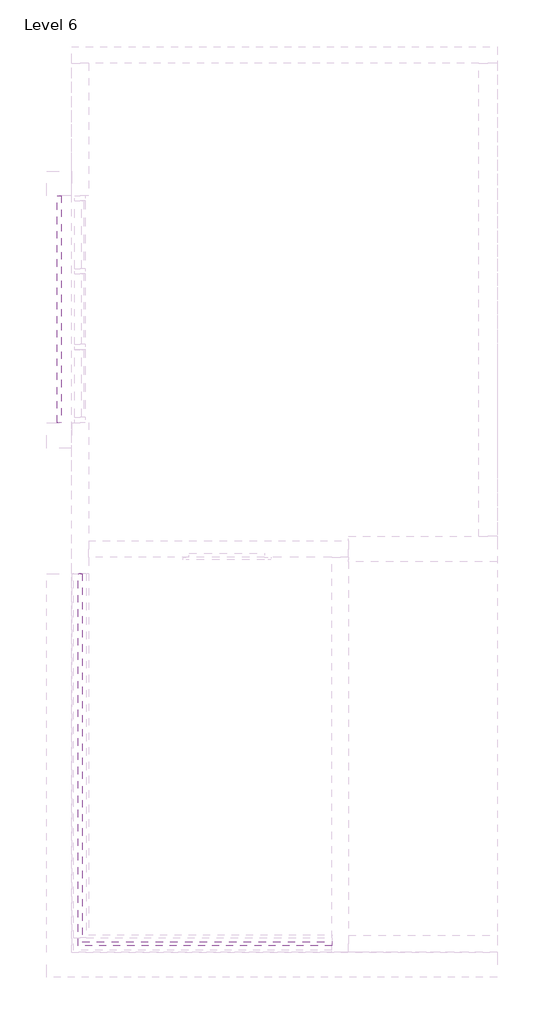
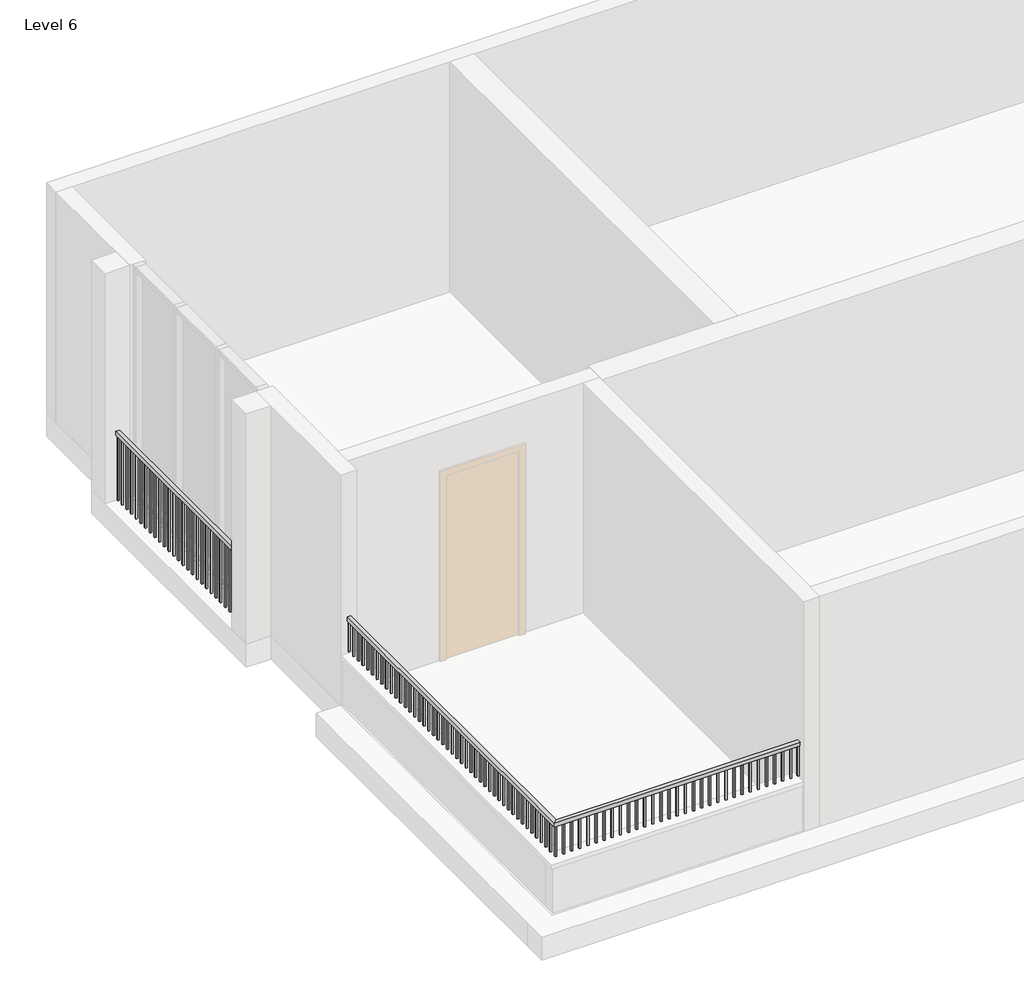
# One storey, part 2 of 2: 2 railings.
"""IFC4 building model written with IfcOpenShell, lengths in millimetres."""

from ifc_helpers import new_model, si_unit, frame, origin, place, context, project, spatial, polyline, outline, extrude, faceted_brep, element, save

model = new_model("IFC4")

# Units and contexts
model_context = context("Model", 3, world=origin())
ifc_project = project(units=[si_unit("LENGTHUNIT", "METRE", prefix="MILLI")], contexts=[model_context])

# Site, building, storey
site = spatial("IfcSite", under=ifc_project)
building = spatial("IfcBuilding", under=site)
storey = spatial("IfcBuildingStorey", under=building, Name="Level 6", Elevation=15240.0)

# Railings
placement = place(None, origin())
element("IfcRailing", 1, ObjectType="Handrail - Rectangular", at=placement, inside=storey, context=model_context, shape_type="SolidModel", body=[
    faceted_brep([(-15179.2169582, -9411.0617616, 17907.0), (-15179.2169582, -9411.0617616, 17856.2), (-15179.2169582, -9360.2617616, 17856.2), (-15179.2169582, -9360.2617616, 17907.0), (-18252.6169582, -9411.0617616, 17907.0), (-18252.6169582, -9411.0617616, 17856.2), (-18201.8169582, -9360.2617616, 17856.2), (-18201.8169582, -9360.2617616, 17907.0), (-18252.6169582, -4908.9117616, 17907.0), (-18201.8169582, -4908.9117616, 17907.0), (-18201.8169582, -4908.9117616, 17856.2), (-18252.6169582, -4908.9117616, 17856.2)], [[[0, 1, 2, 3]], [[1, 0, 4, 5]], [[2, 1, 5, 6]], [[3, 2, 6, 7]], [[0, 3, 7, 4]], [[8, 9, 10, 11]], [[5, 4, 8, 11]], [[6, 5, 11, 10]], [[7, 6, 10, 9]], [[4, 7, 9, 8]]]),
    extrude(outline(polyline([(-18217.6919582, -4924.7867616), (-18236.7419582, -4924.7867616), (-18236.7419582, -4905.7367616), (-18217.6919582, -4905.7367616), (-18217.6919582, -4924.7867616)])), frame((0.0, 0.0, 17449.8), z_axis=(0.0, 0.0, 1.0), x_axis=(1.0, 0.0, 0.0)), (0.0, 0.0, 1.0), 406.4),
    extrude(outline(polyline([(-18217.6919582, -5026.3867616), (-18236.7419582, -5026.3867616), (-18236.7419582, -5007.3367616), (-18217.6919582, -5007.3367616), (-18217.6919582, -5026.3867616)])), frame((0.0, 0.0, 17449.8), z_axis=(0.0, 0.0, 1.0), x_axis=(1.0, 0.0, 0.0)), (0.0, 0.0, 1.0), 406.4),
    extrude(outline(polyline([(-18217.6919582, -5127.9867616), (-18236.7419582, -5127.9867616), (-18236.7419582, -5108.9367616), (-18217.6919582, -5108.9367616), (-18217.6919582, -5127.9867616)])), frame((0.0, 0.0, 17449.8), z_axis=(0.0, 0.0, 1.0), x_axis=(1.0, 0.0, 0.0)), (0.0, 0.0, 1.0), 406.4),
    extrude(outline(polyline([(-18217.6919582, -5229.5867616), (-18236.7419582, -5229.5867616), (-18236.7419582, -5210.5367616), (-18217.6919582, -5210.5367616), (-18217.6919582, -5229.5867616)])), frame((0.0, 0.0, 17449.8), z_axis=(0.0, 0.0, 1.0), x_axis=(1.0, 0.0, 0.0)), (0.0, 0.0, 1.0), 406.4),
    extrude(outline(polyline([(-18217.6919582, -5331.1867616), (-18236.7419582, -5331.1867616), (-18236.7419582, -5312.1367616), (-18217.6919582, -5312.1367616), (-18217.6919582, -5331.1867616)])), frame((0.0, 0.0, 17449.8), z_axis=(0.0, 0.0, 1.0), x_axis=(1.0, 0.0, 0.0)), (0.0, 0.0, 1.0), 406.4),
    extrude(outline(polyline([(-18217.6919582, -5432.7867616), (-18236.7419582, -5432.7867616), (-18236.7419582, -5413.7367616), (-18217.6919582, -5413.7367616), (-18217.6919582, -5432.7867616)])), frame((0.0, 0.0, 17449.8), z_axis=(0.0, 0.0, 1.0), x_axis=(1.0, 0.0, 0.0)), (0.0, 0.0, 1.0), 406.4),
    extrude(outline(polyline([(-18217.6919582, -5534.3867616), (-18236.7419582, -5534.3867616), (-18236.7419582, -5515.3367616), (-18217.6919582, -5515.3367616), (-18217.6919582, -5534.3867616)])), frame((0.0, 0.0, 17449.8), z_axis=(0.0, 0.0, 1.0), x_axis=(1.0, 0.0, 0.0)), (0.0, 0.0, 1.0), 406.4),
    extrude(outline(polyline([(-18217.6919582, -5635.9867616), (-18236.7419582, -5635.9867616), (-18236.7419582, -5616.9367616), (-18217.6919582, -5616.9367616), (-18217.6919582, -5635.9867616)])), frame((0.0, 0.0, 17449.8), z_axis=(0.0, 0.0, 1.0), x_axis=(1.0, 0.0, 0.0)), (0.0, 0.0, 1.0), 406.4),
    extrude(outline(polyline([(-18217.6919582, -5737.5867616), (-18236.7419582, -5737.5867616), (-18236.7419582, -5718.5367616), (-18217.6919582, -5718.5367616), (-18217.6919582, -5737.5867616)])), frame((0.0, 0.0, 17449.8), z_axis=(0.0, 0.0, 1.0), x_axis=(1.0, 0.0, 0.0)), (0.0, 0.0, 1.0), 406.4),
    extrude(outline(polyline([(-18217.6919582, -5839.1867616), (-18236.7419582, -5839.1867616), (-18236.7419582, -5820.1367616), (-18217.6919582, -5820.1367616), (-18217.6919582, -5839.1867616)])), frame((0.0, 0.0, 17449.8), z_axis=(0.0, 0.0, 1.0), x_axis=(1.0, 0.0, 0.0)), (0.0, 0.0, 1.0), 406.4),
    extrude(outline(polyline([(-18217.6919582, -5940.7867616), (-18236.7419582, -5940.7867616), (-18236.7419582, -5921.7367616), (-18217.6919582, -5921.7367616), (-18217.6919582, -5940.7867616)])), frame((0.0, 0.0, 17449.8), z_axis=(0.0, 0.0, 1.0), x_axis=(1.0, 0.0, 0.0)), (0.0, 0.0, 1.0), 406.4),
    extrude(outline(polyline([(-18217.6919582, -6042.3867616), (-18236.7419582, -6042.3867616), (-18236.7419582, -6023.3367616), (-18217.6919582, -6023.3367616), (-18217.6919582, -6042.3867616)])), frame((0.0, 0.0, 17449.8), z_axis=(0.0, 0.0, 1.0), x_axis=(1.0, 0.0, 0.0)), (0.0, 0.0, 1.0), 406.4),
    extrude(outline(polyline([(-18217.6919582, -6143.9867616), (-18236.7419582, -6143.9867616), (-18236.7419582, -6124.9367616), (-18217.6919582, -6124.9367616), (-18217.6919582, -6143.9867616)])), frame((0.0, 0.0, 17449.8), z_axis=(0.0, 0.0, 1.0), x_axis=(1.0, 0.0, 0.0)), (0.0, 0.0, 1.0), 406.4),
    extrude(outline(polyline([(-18217.6919582, -6245.5867616), (-18236.7419582, -6245.5867616), (-18236.7419582, -6226.5367616), (-18217.6919582, -6226.5367616), (-18217.6919582, -6245.5867616)])), frame((0.0, 0.0, 17449.8), z_axis=(0.0, 0.0, 1.0), x_axis=(1.0, 0.0, 0.0)), (0.0, 0.0, 1.0), 406.4),
    extrude(outline(polyline([(-18217.6919582, -6347.1867616), (-18236.7419582, -6347.1867616), (-18236.7419582, -6328.1367616), (-18217.6919582, -6328.1367616), (-18217.6919582, -6347.1867616)])), frame((0.0, 0.0, 17449.8), z_axis=(0.0, 0.0, 1.0), x_axis=(1.0, 0.0, 0.0)), (0.0, 0.0, 1.0), 406.4),
    extrude(outline(polyline([(-18217.6919582, -6448.7867616), (-18236.7419582, -6448.7867616), (-18236.7419582, -6429.7367616), (-18217.6919582, -6429.7367616), (-18217.6919582, -6448.7867616)])), frame((0.0, 0.0, 17449.8), z_axis=(0.0, 0.0, 1.0), x_axis=(1.0, 0.0, 0.0)), (0.0, 0.0, 1.0), 406.4),
    extrude(outline(polyline([(-18217.6919582, -6550.3867616), (-18236.7419582, -6550.3867616), (-18236.7419582, -6531.3367616), (-18217.6919582, -6531.3367616), (-18217.6919582, -6550.3867616)])), frame((0.0, 0.0, 17449.8), z_axis=(0.0, 0.0, 1.0), x_axis=(1.0, 0.0, 0.0)), (0.0, 0.0, 1.0), 406.4),
    extrude(outline(polyline([(-18217.6919582, -6651.9867616), (-18236.7419582, -6651.9867616), (-18236.7419582, -6632.9367616), (-18217.6919582, -6632.9367616), (-18217.6919582, -6651.9867616)])), frame((0.0, 0.0, 17449.8), z_axis=(0.0, 0.0, 1.0), x_axis=(1.0, 0.0, 0.0)), (0.0, 0.0, 1.0), 406.4),
    extrude(outline(polyline([(-18217.6919582, -6753.5867616), (-18236.7419582, -6753.5867616), (-18236.7419582, -6734.5367616), (-18217.6919582, -6734.5367616), (-18217.6919582, -6753.5867616)])), frame((0.0, 0.0, 17449.8), z_axis=(0.0, 0.0, 1.0), x_axis=(1.0, 0.0, 0.0)), (0.0, 0.0, 1.0), 406.4),
    extrude(outline(polyline([(-18217.6919582, -6855.1867616), (-18236.7419582, -6855.1867616), (-18236.7419582, -6836.1367616), (-18217.6919582, -6836.1367616), (-18217.6919582, -6855.1867616)])), frame((0.0, 0.0, 17449.8), z_axis=(0.0, 0.0, 1.0), x_axis=(1.0, 0.0, 0.0)), (0.0, 0.0, 1.0), 406.4),
    extrude(outline(polyline([(-18217.6919582, -6956.7867616), (-18236.7419582, -6956.7867616), (-18236.7419582, -6937.7367616), (-18217.6919582, -6937.7367616), (-18217.6919582, -6956.7867616)])), frame((0.0, 0.0, 17449.8), z_axis=(0.0, 0.0, 1.0), x_axis=(1.0, 0.0, 0.0)), (0.0, 0.0, 1.0), 406.4),
    extrude(outline(polyline([(-18217.6919582, -7058.3867616), (-18236.7419582, -7058.3867616), (-18236.7419582, -7039.3367616), (-18217.6919582, -7039.3367616), (-18217.6919582, -7058.3867616)])), frame((0.0, 0.0, 17449.8), z_axis=(0.0, 0.0, 1.0), x_axis=(1.0, 0.0, 0.0)), (0.0, 0.0, 1.0), 406.4),
    extrude(outline(polyline([(-18217.6919582, -7159.9867616), (-18236.7419582, -7159.9867616), (-18236.7419582, -7140.9367616), (-18217.6919582, -7140.9367616), (-18217.6919582, -7159.9867616)])), frame((0.0, 0.0, 17449.8), z_axis=(0.0, 0.0, 1.0), x_axis=(1.0, 0.0, 0.0)), (0.0, 0.0, 1.0), 406.4),
    extrude(outline(polyline([(-18217.6919582, -7261.5867616), (-18236.7419582, -7261.5867616), (-18236.7419582, -7242.5367616), (-18217.6919582, -7242.5367616), (-18217.6919582, -7261.5867616)])), frame((0.0, 0.0, 17449.8), z_axis=(0.0, 0.0, 1.0), x_axis=(1.0, 0.0, 0.0)), (0.0, 0.0, 1.0), 406.4),
    extrude(outline(polyline([(-18217.6919582, -7363.1867616), (-18236.7419582, -7363.1867616), (-18236.7419582, -7344.1367616), (-18217.6919582, -7344.1367616), (-18217.6919582, -7363.1867616)])), frame((0.0, 0.0, 17449.8), z_axis=(0.0, 0.0, 1.0), x_axis=(1.0, 0.0, 0.0)), (0.0, 0.0, 1.0), 406.4),
    extrude(outline(polyline([(-18217.6919582, -7464.7867616), (-18236.7419582, -7464.7867616), (-18236.7419582, -7445.7367616), (-18217.6919582, -7445.7367616), (-18217.6919582, -7464.7867616)])), frame((0.0, 0.0, 17449.8), z_axis=(0.0, 0.0, 1.0), x_axis=(1.0, 0.0, 0.0)), (0.0, 0.0, 1.0), 406.4),
    extrude(outline(polyline([(-18217.6919582, -7566.3867616), (-18236.7419582, -7566.3867616), (-18236.7419582, -7547.3367616), (-18217.6919582, -7547.3367616), (-18217.6919582, -7566.3867616)])), frame((0.0, 0.0, 17449.8), z_axis=(0.0, 0.0, 1.0), x_axis=(1.0, 0.0, 0.0)), (0.0, 0.0, 1.0), 406.4),
    extrude(outline(polyline([(-18217.6919582, -7667.9867616), (-18236.7419582, -7667.9867616), (-18236.7419582, -7648.9367616), (-18217.6919582, -7648.9367616), (-18217.6919582, -7667.9867616)])), frame((0.0, 0.0, 17449.8), z_axis=(0.0, 0.0, 1.0), x_axis=(1.0, 0.0, 0.0)), (0.0, 0.0, 1.0), 406.4),
    extrude(outline(polyline([(-18217.6919582, -7769.5867616), (-18236.7419582, -7769.5867616), (-18236.7419582, -7750.5367616), (-18217.6919582, -7750.5367616), (-18217.6919582, -7769.5867616)])), frame((0.0, 0.0, 17449.8), z_axis=(0.0, 0.0, 1.0), x_axis=(1.0, 0.0, 0.0)), (0.0, 0.0, 1.0), 406.4),
    extrude(outline(polyline([(-18217.6919582, -7871.1867616), (-18236.7419582, -7871.1867616), (-18236.7419582, -7852.1367616), (-18217.6919582, -7852.1367616), (-18217.6919582, -7871.1867616)])), frame((0.0, 0.0, 17449.8), z_axis=(0.0, 0.0, 1.0), x_axis=(1.0, 0.0, 0.0)), (0.0, 0.0, 1.0), 406.4),
    extrude(outline(polyline([(-18217.6919582, -7972.7867616), (-18236.7419582, -7972.7867616), (-18236.7419582, -7953.7367616), (-18217.6919582, -7953.7367616), (-18217.6919582, -7972.7867616)])), frame((0.0, 0.0, 17449.8), z_axis=(0.0, 0.0, 1.0), x_axis=(1.0, 0.0, 0.0)), (0.0, 0.0, 1.0), 406.4),
    extrude(outline(polyline([(-18217.6919582, -8074.3867616), (-18236.7419582, -8074.3867616), (-18236.7419582, -8055.3367616), (-18217.6919582, -8055.3367616), (-18217.6919582, -8074.3867616)])), frame((0.0, 0.0, 17449.8), z_axis=(0.0, 0.0, 1.0), x_axis=(1.0, 0.0, 0.0)), (0.0, 0.0, 1.0), 406.4),
    extrude(outline(polyline([(-18217.6919582, -8175.9867616), (-18236.7419582, -8175.9867616), (-18236.7419582, -8156.9367616), (-18217.6919582, -8156.9367616), (-18217.6919582, -8175.9867616)])), frame((0.0, 0.0, 17449.8), z_axis=(0.0, 0.0, 1.0), x_axis=(1.0, 0.0, 0.0)), (0.0, 0.0, 1.0), 406.4),
    extrude(outline(polyline([(-18217.6919582, -8277.5867616), (-18236.7419582, -8277.5867616), (-18236.7419582, -8258.5367616), (-18217.6919582, -8258.5367616), (-18217.6919582, -8277.5867616)])), frame((0.0, 0.0, 17449.8), z_axis=(0.0, 0.0, 1.0), x_axis=(1.0, 0.0, 0.0)), (0.0, 0.0, 1.0), 406.4),
    extrude(outline(polyline([(-18217.6919582, -8379.1867616), (-18236.7419582, -8379.1867616), (-18236.7419582, -8360.1367616), (-18217.6919582, -8360.1367616), (-18217.6919582, -8379.1867616)])), frame((0.0, 0.0, 17449.8), z_axis=(0.0, 0.0, 1.0), x_axis=(1.0, 0.0, 0.0)), (0.0, 0.0, 1.0), 406.4),
    extrude(outline(polyline([(-18217.6919582, -8480.7867616), (-18236.7419582, -8480.7867616), (-18236.7419582, -8461.7367616), (-18217.6919582, -8461.7367616), (-18217.6919582, -8480.7867616)])), frame((0.0, 0.0, 17449.8), z_axis=(0.0, 0.0, 1.0), x_axis=(1.0, 0.0, 0.0)), (0.0, 0.0, 1.0), 406.4),
    extrude(outline(polyline([(-18217.6919582, -8582.3867616), (-18236.7419582, -8582.3867616), (-18236.7419582, -8563.3367616), (-18217.6919582, -8563.3367616), (-18217.6919582, -8582.3867616)])), frame((0.0, 0.0, 17449.8), z_axis=(0.0, 0.0, 1.0), x_axis=(1.0, 0.0, 0.0)), (0.0, 0.0, 1.0), 406.4),
    extrude(outline(polyline([(-18217.6919582, -8683.9867616), (-18236.7419582, -8683.9867616), (-18236.7419582, -8664.9367616), (-18217.6919582, -8664.9367616), (-18217.6919582, -8683.9867616)])), frame((0.0, 0.0, 17449.8), z_axis=(0.0, 0.0, 1.0), x_axis=(1.0, 0.0, 0.0)), (0.0, 0.0, 1.0), 406.4),
    extrude(outline(polyline([(-18217.6919582, -8785.5867616), (-18236.7419582, -8785.5867616), (-18236.7419582, -8766.5367616), (-18217.6919582, -8766.5367616), (-18217.6919582, -8785.5867616)])), frame((0.0, 0.0, 17449.8), z_axis=(0.0, 0.0, 1.0), x_axis=(1.0, 0.0, 0.0)), (0.0, 0.0, 1.0), 406.4),
    extrude(outline(polyline([(-18217.6919582, -8887.1867616), (-18236.7419582, -8887.1867616), (-18236.7419582, -8868.1367616), (-18217.6919582, -8868.1367616), (-18217.6919582, -8887.1867616)])), frame((0.0, 0.0, 17449.8), z_axis=(0.0, 0.0, 1.0), x_axis=(1.0, 0.0, 0.0)), (0.0, 0.0, 1.0), 406.4),
    extrude(outline(polyline([(-18217.6919582, -8988.7867616), (-18236.7419582, -8988.7867616), (-18236.7419582, -8969.7367616), (-18217.6919582, -8969.7367616), (-18217.6919582, -8988.7867616)])), frame((0.0, 0.0, 17449.8), z_axis=(0.0, 0.0, 1.0), x_axis=(1.0, 0.0, 0.0)), (0.0, 0.0, 1.0), 406.4),
    extrude(outline(polyline([(-18217.6919582, -9090.3867616), (-18236.7419582, -9090.3867616), (-18236.7419582, -9071.3367616), (-18217.6919582, -9071.3367616), (-18217.6919582, -9090.3867616)])), frame((0.0, 0.0, 17449.8), z_axis=(0.0, 0.0, 1.0), x_axis=(1.0, 0.0, 0.0)), (0.0, 0.0, 1.0), 406.4),
    extrude(outline(polyline([(-18217.6919582, -9191.9867616), (-18236.7419582, -9191.9867616), (-18236.7419582, -9172.9367616), (-18217.6919582, -9172.9367616), (-18217.6919582, -9191.9867616)])), frame((0.0, 0.0, 17449.8), z_axis=(0.0, 0.0, 1.0), x_axis=(1.0, 0.0, 0.0)), (0.0, 0.0, 1.0), 406.4),
    extrude(outline(polyline([(-18217.6919582, -9293.5867616), (-18236.7419582, -9293.5867616), (-18236.7419582, -9274.5367616), (-18217.6919582, -9274.5367616), (-18217.6919582, -9293.5867616)])), frame((0.0, 0.0, 17449.8), z_axis=(0.0, 0.0, 1.0), x_axis=(1.0, 0.0, 0.0)), (0.0, 0.0, 1.0), 406.4),
    extrude(outline(polyline([(-18116.0919582, -9376.1367616), (-18116.0919582, -9395.1867616), (-18135.1419582, -9395.1867616), (-18135.1419582, -9376.1367616), (-18116.0919582, -9376.1367616)])), frame((0.0, 0.0, 17449.8), z_axis=(0.0, 0.0, 1.0), x_axis=(1.0, 0.0, 0.0)), (0.0, 0.0, 1.0), 406.4),
    extrude(outline(polyline([(-18014.4919582, -9376.1367616), (-18014.4919582, -9395.1867616), (-18033.5419582, -9395.1867616), (-18033.5419582, -9376.1367616), (-18014.4919582, -9376.1367616)])), frame((0.0, 0.0, 17449.8), z_axis=(0.0, 0.0, 1.0), x_axis=(1.0, 0.0, 0.0)), (0.0, 0.0, 1.0), 406.4),
    extrude(outline(polyline([(-17912.8919582, -9376.1367616), (-17912.8919582, -9395.1867616), (-17931.9419582, -9395.1867616), (-17931.9419582, -9376.1367616), (-17912.8919582, -9376.1367616)])), frame((0.0, 0.0, 17449.8), z_axis=(0.0, 0.0, 1.0), x_axis=(1.0, 0.0, 0.0)), (0.0, 0.0, 1.0), 406.4),
    extrude(outline(polyline([(-17811.2919582, -9376.1367616), (-17811.2919582, -9395.1867616), (-17830.3419582, -9395.1867616), (-17830.3419582, -9376.1367616), (-17811.2919582, -9376.1367616)])), frame((0.0, 0.0, 17449.8), z_axis=(0.0, 0.0, 1.0), x_axis=(1.0, 0.0, 0.0)), (0.0, 0.0, 1.0), 406.4),
    extrude(outline(polyline([(-17709.6919582, -9376.1367616), (-17709.6919582, -9395.1867616), (-17728.7419582, -9395.1867616), (-17728.7419582, -9376.1367616), (-17709.6919582, -9376.1367616)])), frame((0.0, 0.0, 17449.8), z_axis=(0.0, 0.0, 1.0), x_axis=(1.0, 0.0, 0.0)), (0.0, 0.0, 1.0), 406.4),
    extrude(outline(polyline([(-17608.0919582, -9376.1367616), (-17608.0919582, -9395.1867616), (-17627.1419582, -9395.1867616), (-17627.1419582, -9376.1367616), (-17608.0919582, -9376.1367616)])), frame((0.0, 0.0, 17449.8), z_axis=(0.0, 0.0, 1.0), x_axis=(1.0, 0.0, 0.0)), (0.0, 0.0, 1.0), 406.4),
    extrude(outline(polyline([(-17506.4919582, -9376.1367616), (-17506.4919582, -9395.1867616), (-17525.5419582, -9395.1867616), (-17525.5419582, -9376.1367616), (-17506.4919582, -9376.1367616)])), frame((0.0, 0.0, 17449.8), z_axis=(0.0, 0.0, 1.0), x_axis=(1.0, 0.0, 0.0)), (0.0, 0.0, 1.0), 406.4),
    extrude(outline(polyline([(-17404.8919582, -9376.1367616), (-17404.8919582, -9395.1867616), (-17423.9419582, -9395.1867616), (-17423.9419582, -9376.1367616), (-17404.8919582, -9376.1367616)])), frame((0.0, 0.0, 17449.8), z_axis=(0.0, 0.0, 1.0), x_axis=(1.0, 0.0, 0.0)), (0.0, 0.0, 1.0), 406.4),
    extrude(outline(polyline([(-17303.2919582, -9376.1367616), (-17303.2919582, -9395.1867616), (-17322.3419582, -9395.1867616), (-17322.3419582, -9376.1367616), (-17303.2919582, -9376.1367616)])), frame((0.0, 0.0, 17449.8), z_axis=(0.0, 0.0, 1.0), x_axis=(1.0, 0.0, 0.0)), (0.0, 0.0, 1.0), 406.4),
    extrude(outline(polyline([(-17201.6919582, -9376.1367616), (-17201.6919582, -9395.1867616), (-17220.7419582, -9395.1867616), (-17220.7419582, -9376.1367616), (-17201.6919582, -9376.1367616)])), frame((0.0, 0.0, 17449.8), z_axis=(0.0, 0.0, 1.0), x_axis=(1.0, 0.0, 0.0)), (0.0, 0.0, 1.0), 406.4),
    extrude(outline(polyline([(-17100.0919582, -9376.1367616), (-17100.0919582, -9395.1867616), (-17119.1419582, -9395.1867616), (-17119.1419582, -9376.1367616), (-17100.0919582, -9376.1367616)])), frame((0.0, 0.0, 17449.8), z_axis=(0.0, 0.0, 1.0), x_axis=(1.0, 0.0, 0.0)), (0.0, 0.0, 1.0), 406.4),
    extrude(outline(polyline([(-16998.4919582, -9376.1367616), (-16998.4919582, -9395.1867616), (-17017.5419582, -9395.1867616), (-17017.5419582, -9376.1367616), (-16998.4919582, -9376.1367616)])), frame((0.0, 0.0, 17449.8), z_axis=(0.0, 0.0, 1.0), x_axis=(1.0, 0.0, 0.0)), (0.0, 0.0, 1.0), 406.4),
    extrude(outline(polyline([(-16896.8919582, -9376.1367616), (-16896.8919582, -9395.1867616), (-16915.9419582, -9395.1867616), (-16915.9419582, -9376.1367616), (-16896.8919582, -9376.1367616)])), frame((0.0, 0.0, 17449.8), z_axis=(0.0, 0.0, 1.0), x_axis=(1.0, 0.0, 0.0)), (0.0, 0.0, 1.0), 406.4),
    extrude(outline(polyline([(-16795.2919582, -9376.1367616), (-16795.2919582, -9395.1867616), (-16814.3419582, -9395.1867616), (-16814.3419582, -9376.1367616), (-16795.2919582, -9376.1367616)])), frame((0.0, 0.0, 17449.8), z_axis=(0.0, 0.0, 1.0), x_axis=(1.0, 0.0, 0.0)), (0.0, 0.0, 1.0), 406.4),
    extrude(outline(polyline([(-16693.6919582, -9376.1367616), (-16693.6919582, -9395.1867616), (-16712.7419582, -9395.1867616), (-16712.7419582, -9376.1367616), (-16693.6919582, -9376.1367616)])), frame((0.0, 0.0, 17449.8), z_axis=(0.0, 0.0, 1.0), x_axis=(1.0, 0.0, 0.0)), (0.0, 0.0, 1.0), 406.4),
    extrude(outline(polyline([(-16592.0919582, -9376.1367616), (-16592.0919582, -9395.1867616), (-16611.1419582, -9395.1867616), (-16611.1419582, -9376.1367616), (-16592.0919582, -9376.1367616)])), frame((0.0, 0.0, 17449.8), z_axis=(0.0, 0.0, 1.0), x_axis=(1.0, 0.0, 0.0)), (0.0, 0.0, 1.0), 406.4),
    extrude(outline(polyline([(-16490.4919582, -9376.1367616), (-16490.4919582, -9395.1867616), (-16509.5419582, -9395.1867616), (-16509.5419582, -9376.1367616), (-16490.4919582, -9376.1367616)])), frame((0.0, 0.0, 17449.8), z_axis=(0.0, 0.0, 1.0), x_axis=(1.0, 0.0, 0.0)), (0.0, 0.0, 1.0), 406.4),
    extrude(outline(polyline([(-16388.8919582, -9376.1367616), (-16388.8919582, -9395.1867616), (-16407.9419582, -9395.1867616), (-16407.9419582, -9376.1367616), (-16388.8919582, -9376.1367616)])), frame((0.0, 0.0, 17449.8), z_axis=(0.0, 0.0, 1.0), x_axis=(1.0, 0.0, 0.0)), (0.0, 0.0, 1.0), 406.4),
    extrude(outline(polyline([(-16287.2919582, -9376.1367616), (-16287.2919582, -9395.1867616), (-16306.3419582, -9395.1867616), (-16306.3419582, -9376.1367616), (-16287.2919582, -9376.1367616)])), frame((0.0, 0.0, 17449.8), z_axis=(0.0, 0.0, 1.0), x_axis=(1.0, 0.0, 0.0)), (0.0, 0.0, 1.0), 406.4),
    extrude(outline(polyline([(-16185.6919582, -9376.1367616), (-16185.6919582, -9395.1867616), (-16204.7419582, -9395.1867616), (-16204.7419582, -9376.1367616), (-16185.6919582, -9376.1367616)])), frame((0.0, 0.0, 17449.8), z_axis=(0.0, 0.0, 1.0), x_axis=(1.0, 0.0, 0.0)), (0.0, 0.0, 1.0), 406.4),
    extrude(outline(polyline([(-16084.0919582, -9376.1367616), (-16084.0919582, -9395.1867616), (-16103.1419582, -9395.1867616), (-16103.1419582, -9376.1367616), (-16084.0919582, -9376.1367616)])), frame((0.0, 0.0, 17449.8), z_axis=(0.0, 0.0, 1.0), x_axis=(1.0, 0.0, 0.0)), (0.0, 0.0, 1.0), 406.4),
    extrude(outline(polyline([(-15982.4919582, -9376.1367616), (-15982.4919582, -9395.1867616), (-16001.5419582, -9395.1867616), (-16001.5419582, -9376.1367616), (-15982.4919582, -9376.1367616)])), frame((0.0, 0.0, 17449.8), z_axis=(0.0, 0.0, 1.0), x_axis=(1.0, 0.0, 0.0)), (0.0, 0.0, 1.0), 406.4),
    extrude(outline(polyline([(-15880.8919582, -9376.1367616), (-15880.8919582, -9395.1867616), (-15899.9419582, -9395.1867616), (-15899.9419582, -9376.1367616), (-15880.8919582, -9376.1367616)])), frame((0.0, 0.0, 17449.8), z_axis=(0.0, 0.0, 1.0), x_axis=(1.0, 0.0, 0.0)), (0.0, 0.0, 1.0), 406.4),
    extrude(outline(polyline([(-15779.2919582, -9376.1367616), (-15779.2919582, -9395.1867616), (-15798.3419582, -9395.1867616), (-15798.3419582, -9376.1367616), (-15779.2919582, -9376.1367616)])), frame((0.0, 0.0, 17449.8), z_axis=(0.0, 0.0, 1.0), x_axis=(1.0, 0.0, 0.0)), (0.0, 0.0, 1.0), 406.4),
    extrude(outline(polyline([(-15677.6919582, -9376.1367616), (-15677.6919582, -9395.1867616), (-15696.7419582, -9395.1867616), (-15696.7419582, -9376.1367616), (-15677.6919582, -9376.1367616)])), frame((0.0, 0.0, 17449.8), z_axis=(0.0, 0.0, 1.0), x_axis=(1.0, 0.0, 0.0)), (0.0, 0.0, 1.0), 406.4),
    extrude(outline(polyline([(-15576.0919582, -9376.1367616), (-15576.0919582, -9395.1867616), (-15595.1419582, -9395.1867616), (-15595.1419582, -9376.1367616), (-15576.0919582, -9376.1367616)])), frame((0.0, 0.0, 17449.8), z_axis=(0.0, 0.0, 1.0), x_axis=(1.0, 0.0, 0.0)), (0.0, 0.0, 1.0), 406.4),
    extrude(outline(polyline([(-15474.4919582, -9376.1367616), (-15474.4919582, -9395.1867616), (-15493.5419582, -9395.1867616), (-15493.5419582, -9376.1367616), (-15474.4919582, -9376.1367616)])), frame((0.0, 0.0, 17449.8), z_axis=(0.0, 0.0, 1.0), x_axis=(1.0, 0.0, 0.0)), (0.0, 0.0, 1.0), 406.4),
    extrude(outline(polyline([(-15372.8919582, -9376.1367616), (-15372.8919582, -9395.1867616), (-15391.9419582, -9395.1867616), (-15391.9419582, -9376.1367616), (-15372.8919582, -9376.1367616)])), frame((0.0, 0.0, 17449.8), z_axis=(0.0, 0.0, 1.0), x_axis=(1.0, 0.0, 0.0)), (0.0, 0.0, 1.0), 406.4),
    extrude(outline(polyline([(-15271.2919582, -9376.1367616), (-15271.2919582, -9395.1867616), (-15290.3419582, -9395.1867616), (-15290.3419582, -9376.1367616), (-15271.2919582, -9376.1367616)])), frame((0.0, 0.0, 17449.8), z_axis=(0.0, 0.0, 1.0), x_axis=(1.0, 0.0, 0.0)), (0.0, 0.0, 1.0), 406.4),
    extrude(outline(polyline([(-18217.6919582, -9376.1367616), (-18217.6919582, -9395.1867616), (-18236.7419582, -9395.1867616), (-18236.7419582, -9376.1367616), (-18217.6919582, -9376.1367616)])), frame((0.0, 0.0, 17449.8), z_axis=(0.0, 0.0, 1.0), x_axis=(1.0, 0.0, 0.0)), (0.0, 0.0, 1.0), 406.4),
    extrude(outline(polyline([(-18217.6919582, -4927.9617616), (-18236.7419582, -4927.9617616), (-18236.7419582, -4908.9117616), (-18217.6919582, -4908.9117616), (-18217.6919582, -4927.9617616)])), frame((0.0, 0.0, 17449.8), z_axis=(0.0, 0.0, 1.0), x_axis=(1.0, 0.0, 0.0)), (0.0, 0.0, 1.0), 406.4),
    extrude(outline(polyline([(-15179.2169582, -9376.1367616), (-15179.2169582, -9395.1867616), (-15198.2669582, -9395.1867616), (-15198.2669582, -9376.1367616), (-15179.2169582, -9376.1367616)])), frame((0.0, 0.0, 17449.8), z_axis=(0.0, 0.0, 1.0), x_axis=(1.0, 0.0, 0.0)), (0.0, 0.0, 1.0), 406.4),
])
element("IfcRailing", 2, ObjectType="Handrail - Rectangular 2", at=placement, inside=storey, context=model_context, shape_type="SweptSolid", body=[
    extrude(outline(polyline([(-18506.6169582, -336.9117616), (-18455.8169582, -336.9117616), (-18455.8169582, -3080.1117616), (-18506.6169582, -3080.1117616), (-18506.6169582, -336.9117616)])), frame((0.0, 0.0, 17627.6), z_axis=(0.0, 0.0, 1.0), x_axis=(1.0, 0.0, 0.0)), (0.0, 0.0, 1.0), 50.8),
    extrude(outline(polyline([(-18490.7419582, -2968.9867616), (-18471.6919582, -2968.9867616), (-18471.6919582, -2988.0367616), (-18490.7419582, -2988.0367616), (-18490.7419582, -2968.9867616)])), frame((0.0, 0.0, 16764.0), z_axis=(0.0, 0.0, 1.0), x_axis=(1.0, 0.0, 0.0)), (0.0, 0.0, 1.0), 863.6),
    extrude(outline(polyline([(-18490.7419582, -2867.3867616), (-18471.6919582, -2867.3867616), (-18471.6919582, -2886.4367616), (-18490.7419582, -2886.4367616), (-18490.7419582, -2867.3867616)])), frame((0.0, 0.0, 16764.0), z_axis=(0.0, 0.0, 1.0), x_axis=(1.0, 0.0, 0.0)), (0.0, 0.0, 1.0), 863.6),
    extrude(outline(polyline([(-18490.7419582, -2765.7867616), (-18471.6919582, -2765.7867616), (-18471.6919582, -2784.8367616), (-18490.7419582, -2784.8367616), (-18490.7419582, -2765.7867616)])), frame((0.0, 0.0, 16764.0), z_axis=(0.0, 0.0, 1.0), x_axis=(1.0, 0.0, 0.0)), (0.0, 0.0, 1.0), 863.6),
    extrude(outline(polyline([(-18490.7419582, -2664.1867616), (-18471.6919582, -2664.1867616), (-18471.6919582, -2683.2367616), (-18490.7419582, -2683.2367616), (-18490.7419582, -2664.1867616)])), frame((0.0, 0.0, 16764.0), z_axis=(0.0, 0.0, 1.0), x_axis=(1.0, 0.0, 0.0)), (0.0, 0.0, 1.0), 863.6),
    extrude(outline(polyline([(-18490.7419582, -2562.5867616), (-18471.6919582, -2562.5867616), (-18471.6919582, -2581.6367616), (-18490.7419582, -2581.6367616), (-18490.7419582, -2562.5867616)])), frame((0.0, 0.0, 16764.0), z_axis=(0.0, 0.0, 1.0), x_axis=(1.0, 0.0, 0.0)), (0.0, 0.0, 1.0), 863.6),
    extrude(outline(polyline([(-18490.7419582, -2460.9867616), (-18471.6919582, -2460.9867616), (-18471.6919582, -2480.0367616), (-18490.7419582, -2480.0367616), (-18490.7419582, -2460.9867616)])), frame((0.0, 0.0, 16764.0), z_axis=(0.0, 0.0, 1.0), x_axis=(1.0, 0.0, 0.0)), (0.0, 0.0, 1.0), 863.6),
    extrude(outline(polyline([(-18490.7419582, -2359.3867616), (-18471.6919582, -2359.3867616), (-18471.6919582, -2378.4367616), (-18490.7419582, -2378.4367616), (-18490.7419582, -2359.3867616)])), frame((0.0, 0.0, 16764.0), z_axis=(0.0, 0.0, 1.0), x_axis=(1.0, 0.0, 0.0)), (0.0, 0.0, 1.0), 863.6),
    extrude(outline(polyline([(-18490.7419582, -2257.7867616), (-18471.6919582, -2257.7867616), (-18471.6919582, -2276.8367616), (-18490.7419582, -2276.8367616), (-18490.7419582, -2257.7867616)])), frame((0.0, 0.0, 16764.0), z_axis=(0.0, 0.0, 1.0), x_axis=(1.0, 0.0, 0.0)), (0.0, 0.0, 1.0), 863.6),
    extrude(outline(polyline([(-18490.7419582, -2156.1867616), (-18471.6919582, -2156.1867616), (-18471.6919582, -2175.2367616), (-18490.7419582, -2175.2367616), (-18490.7419582, -2156.1867616)])), frame((0.0, 0.0, 16764.0), z_axis=(0.0, 0.0, 1.0), x_axis=(1.0, 0.0, 0.0)), (0.0, 0.0, 1.0), 863.6),
    extrude(outline(polyline([(-18490.7419582, -2054.5867616), (-18471.6919582, -2054.5867616), (-18471.6919582, -2073.6367616), (-18490.7419582, -2073.6367616), (-18490.7419582, -2054.5867616)])), frame((0.0, 0.0, 16764.0), z_axis=(0.0, 0.0, 1.0), x_axis=(1.0, 0.0, 0.0)), (0.0, 0.0, 1.0), 863.6),
    extrude(outline(polyline([(-18490.7419582, -1952.9867616), (-18471.6919582, -1952.9867616), (-18471.6919582, -1972.0367616), (-18490.7419582, -1972.0367616), (-18490.7419582, -1952.9867616)])), frame((0.0, 0.0, 16764.0), z_axis=(0.0, 0.0, 1.0), x_axis=(1.0, 0.0, 0.0)), (0.0, 0.0, 1.0), 863.6),
    extrude(outline(polyline([(-18490.7419582, -1851.3867616), (-18471.6919582, -1851.3867616), (-18471.6919582, -1870.4367616), (-18490.7419582, -1870.4367616), (-18490.7419582, -1851.3867616)])), frame((0.0, 0.0, 16764.0), z_axis=(0.0, 0.0, 1.0), x_axis=(1.0, 0.0, 0.0)), (0.0, 0.0, 1.0), 863.6),
    extrude(outline(polyline([(-18490.7419582, -1749.7867616), (-18471.6919582, -1749.7867616), (-18471.6919582, -1768.8367616), (-18490.7419582, -1768.8367616), (-18490.7419582, -1749.7867616)])), frame((0.0, 0.0, 16764.0), z_axis=(0.0, 0.0, 1.0), x_axis=(1.0, 0.0, 0.0)), (0.0, 0.0, 1.0), 863.6),
    extrude(outline(polyline([(-18490.7419582, -1648.1867616), (-18471.6919582, -1648.1867616), (-18471.6919582, -1667.2367616), (-18490.7419582, -1667.2367616), (-18490.7419582, -1648.1867616)])), frame((0.0, 0.0, 16764.0), z_axis=(0.0, 0.0, 1.0), x_axis=(1.0, 0.0, 0.0)), (0.0, 0.0, 1.0), 863.6),
    extrude(outline(polyline([(-18490.7419582, -1546.5867616), (-18471.6919582, -1546.5867616), (-18471.6919582, -1565.6367616), (-18490.7419582, -1565.6367616), (-18490.7419582, -1546.5867616)])), frame((0.0, 0.0, 16764.0), z_axis=(0.0, 0.0, 1.0), x_axis=(1.0, 0.0, 0.0)), (0.0, 0.0, 1.0), 863.6),
    extrude(outline(polyline([(-18490.7419582, -1444.9867616), (-18471.6919582, -1444.9867616), (-18471.6919582, -1464.0367616), (-18490.7419582, -1464.0367616), (-18490.7419582, -1444.9867616)])), frame((0.0, 0.0, 16764.0), z_axis=(0.0, 0.0, 1.0), x_axis=(1.0, 0.0, 0.0)), (0.0, 0.0, 1.0), 863.6),
    extrude(outline(polyline([(-18490.7419582, -1343.3867616), (-18471.6919582, -1343.3867616), (-18471.6919582, -1362.4367616), (-18490.7419582, -1362.4367616), (-18490.7419582, -1343.3867616)])), frame((0.0, 0.0, 16764.0), z_axis=(0.0, 0.0, 1.0), x_axis=(1.0, 0.0, 0.0)), (0.0, 0.0, 1.0), 863.6),
    extrude(outline(polyline([(-18490.7419582, -1241.7867616), (-18471.6919582, -1241.7867616), (-18471.6919582, -1260.8367616), (-18490.7419582, -1260.8367616), (-18490.7419582, -1241.7867616)])), frame((0.0, 0.0, 16764.0), z_axis=(0.0, 0.0, 1.0), x_axis=(1.0, 0.0, 0.0)), (0.0, 0.0, 1.0), 863.6),
    extrude(outline(polyline([(-18490.7419582, -1140.1867616), (-18471.6919582, -1140.1867616), (-18471.6919582, -1159.2367616), (-18490.7419582, -1159.2367616), (-18490.7419582, -1140.1867616)])), frame((0.0, 0.0, 16764.0), z_axis=(0.0, 0.0, 1.0), x_axis=(1.0, 0.0, 0.0)), (0.0, 0.0, 1.0), 863.6),
    extrude(outline(polyline([(-18490.7419582, -1038.5867616), (-18471.6919582, -1038.5867616), (-18471.6919582, -1057.6367616), (-18490.7419582, -1057.6367616), (-18490.7419582, -1038.5867616)])), frame((0.0, 0.0, 16764.0), z_axis=(0.0, 0.0, 1.0), x_axis=(1.0, 0.0, 0.0)), (0.0, 0.0, 1.0), 863.6),
    extrude(outline(polyline([(-18490.7419582, -936.9867616), (-18471.6919582, -936.9867616), (-18471.6919582, -956.0367616), (-18490.7419582, -956.0367616), (-18490.7419582, -936.9867616)])), frame((0.0, 0.0, 16764.0), z_axis=(0.0, 0.0, 1.0), x_axis=(1.0, 0.0, 0.0)), (0.0, 0.0, 1.0), 863.6),
    extrude(outline(polyline([(-18490.7419582, -835.3867616), (-18471.6919582, -835.3867616), (-18471.6919582, -854.4367616), (-18490.7419582, -854.4367616), (-18490.7419582, -835.3867616)])), frame((0.0, 0.0, 16764.0), z_axis=(0.0, 0.0, 1.0), x_axis=(1.0, 0.0, 0.0)), (0.0, 0.0, 1.0), 863.6),
    extrude(outline(polyline([(-18490.7419582, -733.7867616), (-18471.6919582, -733.7867616), (-18471.6919582, -752.8367616), (-18490.7419582, -752.8367616), (-18490.7419582, -733.7867616)])), frame((0.0, 0.0, 16764.0), z_axis=(0.0, 0.0, 1.0), x_axis=(1.0, 0.0, 0.0)), (0.0, 0.0, 1.0), 863.6),
    extrude(outline(polyline([(-18490.7419582, -632.1867616), (-18471.6919582, -632.1867616), (-18471.6919582, -651.2367616), (-18490.7419582, -651.2367616), (-18490.7419582, -632.1867616)])), frame((0.0, 0.0, 16764.0), z_axis=(0.0, 0.0, 1.0), x_axis=(1.0, 0.0, 0.0)), (0.0, 0.0, 1.0), 863.6),
    extrude(outline(polyline([(-18490.7419582, -530.5867616), (-18471.6919582, -530.5867616), (-18471.6919582, -549.6367616), (-18490.7419582, -549.6367616), (-18490.7419582, -530.5867616)])), frame((0.0, 0.0, 16764.0), z_axis=(0.0, 0.0, 1.0), x_axis=(1.0, 0.0, 0.0)), (0.0, 0.0, 1.0), 863.6),
    extrude(outline(polyline([(-18490.7419582, -428.9867616), (-18471.6919582, -428.9867616), (-18471.6919582, -448.0367616), (-18490.7419582, -448.0367616), (-18490.7419582, -428.9867616)])), frame((0.0, 0.0, 16764.0), z_axis=(0.0, 0.0, 1.0), x_axis=(1.0, 0.0, 0.0)), (0.0, 0.0, 1.0), 863.6),
    extrude(outline(polyline([(-18490.7419582, -3061.0617616), (-18471.6919582, -3061.0617616), (-18471.6919582, -3080.1117616), (-18490.7419582, -3080.1117616), (-18490.7419582, -3061.0617616)])), frame((0.0, 0.0, 16764.0), z_axis=(0.0, 0.0, 1.0), x_axis=(1.0, 0.0, 0.0)), (0.0, 0.0, 1.0), 863.6),
    extrude(outline(polyline([(-18490.7419582, -336.9117616), (-18471.6919582, -336.9117616), (-18471.6919582, -355.9617616), (-18490.7419582, -355.9617616), (-18490.7419582, -336.9117616)])), frame((0.0, 0.0, 16764.0), z_axis=(0.0, 0.0, 1.0), x_axis=(1.0, 0.0, 0.0)), (0.0, 0.0, 1.0), 863.6),
])

save(model, "model.ifc")

# Revit data of these elements
# Type "Handrail - Rectangular"
#   Assembly Code = "C2010400"
#   built-in parameter 1008612 = 0.0416667 (stored number, unit not read)
#   built-in parameter 1008611 = 0.0416667 (stored number, unit not read)
#   built-in parameter 1008609 = 0.333333 (stored number, unit not read)
#   built-in parameter 1008604 = 0.166667 (stored number, unit not read)
#   built-in parameter 1008603 = 0.166667 (stored number, unit not read)
#   Railing Height = 1' - 6"
#   built-in parameter 1008630 = 2
#   built-in parameter 1008610 = 2
#   built-in parameter 1008618 = Baluster - Square : 3/4"
# Type "Handrail - Rectangular 2"
#   Assembly Code = "C2010400"
#   built-in parameter 1008612 = 0.0416667 (stored number, unit not read)
#   built-in parameter 1008611 = 0.0416667 (stored number, unit not read)
#   built-in parameter 1008609 = 0.333333 (stored number, unit not read)
#   built-in parameter 1008604 = 0.166667 (stored number, unit not read)
#   built-in parameter 1008603 = 0.166667 (stored number, unit not read)
#   Railing Height = 3' - 0"
#   built-in parameter 1008630 = 2
#   built-in parameter 1008610 = 2
#   built-in parameter 1008618 = Baluster - Square : 3/4"
# Element 1 (IfcRailing, "Handrail - Rectangular")
#   built-in parameter 1008621 = 7.25 (stored number, unit not read)
#   Phase Created = New Construction
# Element 2 (IfcRailing, "Handrail - Rectangular 2")
#   built-in parameter 1008621 = 5 (stored number, unit not read)
#   Phase Created = New Construction
